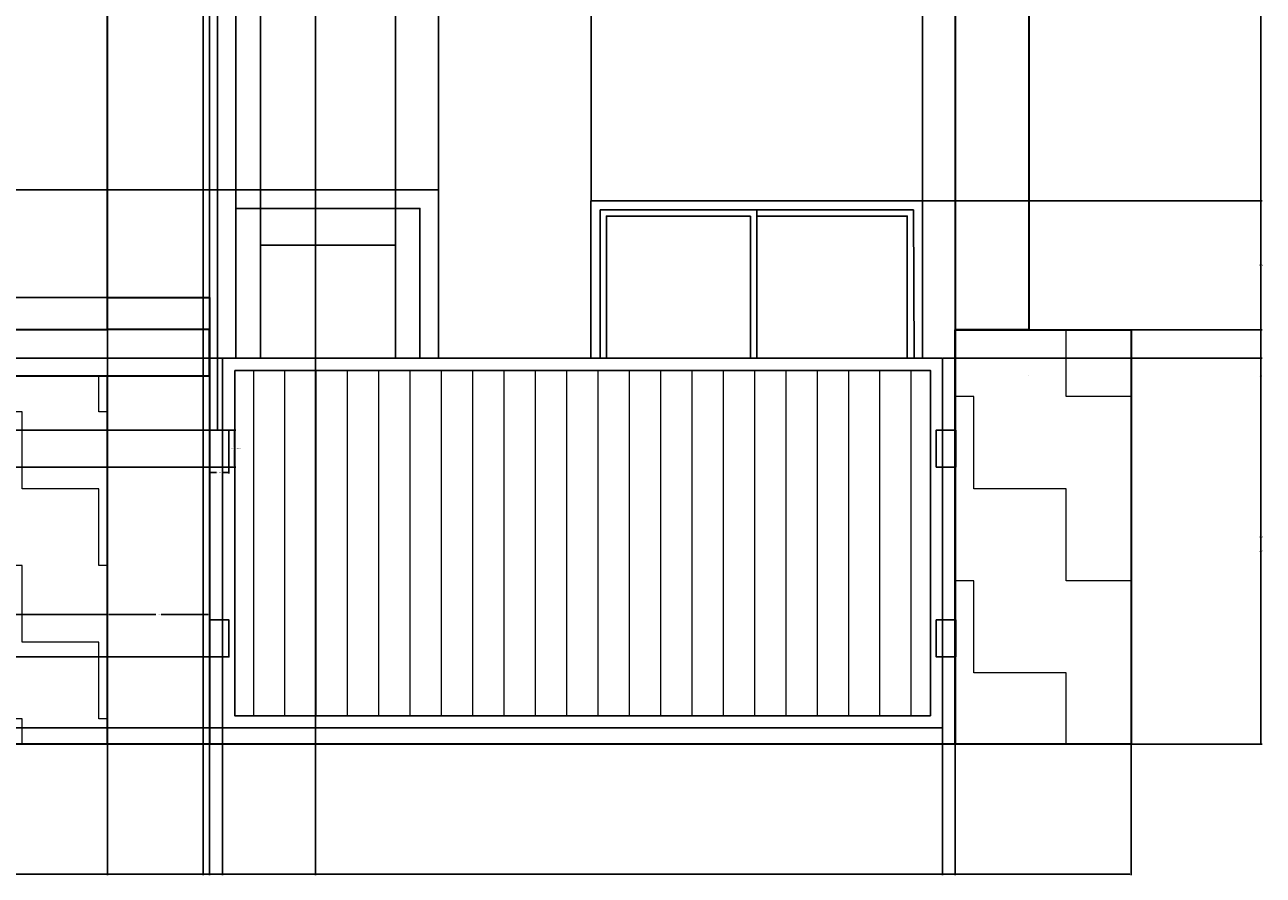
# Model space of a CAD drawing. Units: inches. Extents: x -3 to 302, y -138 to 325.
# Tile 2 of 5: x 100 to 302, y -138 to 1. Entities that reach past the tile are written whole.
import ezdxf

# ---------------------------------------------------------------- set-up
doc = ezdxf.new("R2010")
doc.units = ezdxf.units.IN
doc.header["$MEASUREMENT"] = 0
for name, color, linetype, lineweight in [('A-ANNO-DIMS', 2, 'Continuous', 18), ('A-DOOR', 4, 'Continuous', 25), ('A-ELEV', 7, 'Continuous', 35), ('A-ELEV-PATT', 8, 'Continuous', 13), ('A-GLAZ', 3, 'Continuous', 25)]:
    doc.layers.add(name, color=color, linetype=linetype, lineweight=lineweight)
doc.styles.get("Standard").update_dxf_attribs({"font": 'arial.ttf'})
doc.dimstyles.get("Standard").update_dxf_attribs({"dimtxt": 0.18, "dimasz": 0.18, "dimexe": 0.18, "dimexo": 0.0625, "dimgap": 0.09, "dimtad": 0, "dimtih": 1, "dimtoh": 1, "dimdec": 4, "dimzin": 0, "dimdsep": 46, "dimtxsty": 'Standard', "dimcen": 0.09, "dimadec": 0, "dimazin": 0, "dimtfac": 1, "dimtdec": 4, "dimtofl": 0, "dimtmove": 0, "dimatfit": 3, "dimfxl": 1, "dimtolj": 1, "dimtzin": 0, "dimarcsym": 0})

# ---------------------------------------------------------------- blocks, each defined once
blk = doc.blocks.new('GATE-HINGE')
blk.add_lwpolyline([(130.49, -65.43), (133.68, -65.43), (133.68, -71.46), (130.49, -71.46)], close=True)
blk = doc.blocks.new('*D11')
at = {"layer": 'A-ANNO-DIMS', "color": 0, "lineweight": -2, "transparency": 16777216}
for p, q in [((133.74, -65.43), (134.77, -65.43)), ((134.59, -65.61), (134.59, -68.26)), ((134.59, -71.28), (134.59, -68.62)), ((133.74, -71.46), (134.77, -71.46))]:
    blk.add_line(p, q, dxfattribs=at)
at = {"layer": 'A-ANNO-DIMS', "color": 0, "transparency": 16777216}
for points in [[(134.56, -65.61), (134.62, -65.61), (134.59, -65.43)], [(134.56, -71.28), (134.62, -71.28), (134.59, -71.46)]]:
    blk.add_solid(points, dxfattribs=at)
at = {"layer": 'Defpoints', "color": 0, "transparency": 16777216}
for p in [(133.68, -65.43), (134.59, -65.43), (133.68, -71.46)]:
    blk.add_point(p, dxfattribs=at)
at = {"layer": 'A-ANNO-DIMS', "color": 0, "transparency": 16777216, "insert": (134.59, -68.44), "char_height": 0.18, "attachment_point": 5}
blk.add_mtext('\\A1;GATE HINGE 6 TYP.', dxfattribs=at)
blk = doc.blocks.new('*D12')
at = {"layer": 'A-ANNO-DIMS', "color": 0, "lineweight": -2, "transparency": 16777216}
for p, q in [((130.49, -71.52), (130.49, -72.54)), ((130.67, -72.36), (131.63, -72.36)), ((133.5, -72.36), (132.54, -72.36)), ((133.68, -71.52), (133.68, -72.54))]:
    blk.add_line(p, q, dxfattribs=at)
at = {"layer": 'A-ANNO-DIMS', "color": 0, "transparency": 16777216}
for points in [[(130.67, -72.33), (130.67, -72.39), (130.49, -72.36)], [(133.5, -72.33), (133.5, -72.39), (133.68, -72.36)]]:
    blk.add_solid(points, dxfattribs=at)
at = {"layer": 'Defpoints', "color": 0, "transparency": 16777216}
for p in [(130.49, -71.46), (133.68, -71.46), (133.68, -72.36)]:
    blk.add_point(p, dxfattribs=at)
at = {"layer": 'A-ANNO-DIMS', "color": 0, "transparency": 16777216, "insert": (132.09, -72.36), "char_height": 0.18, "attachment_point": 5}
blk.add_mtext('\\A1;3 TYP.', dxfattribs=at)
blk = doc.blocks.new('*D17')
at = {"layer": 'A-ANNO-DIMS', "color": 0, "lineweight": -2, "transparency": 16777216}
for p, q in [((18.53, -56.69), (18.53, -137.96)), ((280.59, -116.69), (280.59, -137.96)), ((18.71, -137.78), (149.1, -137.78)), ((280.41, -137.78), (150.03, -137.78))]:
    blk.add_line(p, q, dxfattribs=at)
at = {"layer": 'A-ANNO-DIMS', "color": 0, "transparency": 16777216}
for points in [[(18.71, -137.75), (18.71, -137.81), (18.53, -137.78)], [(280.41, -137.75), (280.41, -137.81), (280.59, -137.78)]]:
    blk.add_solid(points, dxfattribs=at)
at = {"layer": 'Defpoints', "color": 0, "transparency": 16777216}
for p in [(18.53, -56.63), (280.59, -116.63), (280.59, -137.78)]:
    blk.add_point(p, dxfattribs=at)
at = {"layer": 'A-ANNO-DIMS', "color": 0, "transparency": 16777216, "insert": (149.56, -137.78), "char_height": 0.18, "attachment_point": 5}
blk.add_mtext('\\A1;262.06', dxfattribs=at)
blk = doc.blocks.new('*D19')
at = {"layer": 'A-ANNO-DIMS', "color": 0, "lineweight": -2, "transparency": 16777216}
for p, q in [((275.98, 3.37), (301.92, 3.37)), ((301.74, 3.19), (301.74, -56.44)), ((301.74, -116.45), (301.74, -56.81)), ((280.66, -116.63), (301.92, -116.63))]:
    blk.add_line(p, q, dxfattribs=at)
at = {"layer": 'A-ANNO-DIMS', "color": 0, "transparency": 16777216}
for points in [[(301.71, 3.19), (301.77, 3.19), (301.74, 3.37)], [(301.71, -116.45), (301.77, -116.45), (301.74, -116.63)]]:
    blk.add_solid(points, dxfattribs=at)
at = {"layer": 'Defpoints', "color": 0, "transparency": 16777216}
for p in [(275.92, 3.37), (301.74, 3.37), (280.59, -116.63)]:
    blk.add_point(p, dxfattribs=at)
at = {"layer": 'A-ANNO-DIMS', "color": 0, "transparency": 16777216, "insert": (301.74, -56.63), "char_height": 0.18, "attachment_point": 5}
blk.add_mtext('\\A1;120', dxfattribs=at)
blk = doc.blocks.new('*D32')
at = {"layer": 'A-ANNO-DIMS', "color": 0, "lineweight": -2, "transparency": 16777216}
for p, q in [((23.92, -116.56), (23.92, -95.3)), ((24.1, -95.48), (68.7, -95.48)), ((113.74, -95.48), (69.14, -95.48)), ((113.92, -116.56), (113.92, -95.3))]:
    blk.add_line(p, q, dxfattribs=at)
at = {"layer": 'A-ANNO-DIMS', "color": 0, "transparency": 16777216}
for points in [[(24.1, -95.45), (24.1, -95.51), (23.92, -95.48)], [(113.74, -95.45), (113.74, -95.51), (113.92, -95.48)]]:
    blk.add_solid(points, dxfattribs=at)
at = {"layer": 'Defpoints', "color": 0, "transparency": 16777216}
for p in [(113.92, -95.48), (23.92, -116.63), (113.92, -116.63)]:
    blk.add_point(p, dxfattribs=at)
at = {"layer": 'A-ANNO-DIMS', "color": 0, "transparency": 16777216, "insert": (68.92, -95.48), "char_height": 0.18, "attachment_point": 5}
blk.add_mtext('\\A1;90', dxfattribs=at)
blk = doc.blocks.new('*D33')
at = {"layer": 'A-ANNO-DIMS', "color": 0, "lineweight": -2, "transparency": 16777216}
for p, q in [((113.92, -116.56), (113.92, -95.3)), ((114.1, -95.48), (121.75, -95.48)), ((130.31, -95.48), (122.66, -95.48)), ((130.49, -116.56), (130.49, -95.3))]:
    blk.add_line(p, q, dxfattribs=at)
at = {"layer": 'A-ANNO-DIMS', "color": 0, "transparency": 16777216}
for points in [[(114.1, -95.45), (114.1, -95.51), (113.92, -95.48)], [(130.31, -95.45), (130.31, -95.51), (130.49, -95.48)]]:
    blk.add_solid(points, dxfattribs=at)
at = {"layer": 'Defpoints', "color": 0, "transparency": 16777216}
for p in [(130.49, -95.48), (113.92, -116.63), (130.49, -116.63)]:
    blk.add_point(p, dxfattribs=at)
at = {"layer": 'A-ANNO-DIMS', "color": 0, "transparency": 16777216, "insert": (122.21, -95.48), "char_height": 0.18, "attachment_point": 5}
blk.add_mtext('\\A1;16.567', dxfattribs=at)
blk = doc.blocks.new('*D66')
at = {"layer": 'A-ANNO-DIMS', "color": 0, "lineweight": -2, "transparency": 16777216}
for p, q in [((113.92, 141.31), (113.92, -137.96)), ((129.47, 141.31), (129.47, -137.96)), ((114.1, -137.78), (121.24, -137.78)), ((129.29, -137.78), (122.15, -137.78))]:
    blk.add_line(p, q, dxfattribs=at)
at = {"layer": 'A-ANNO-DIMS', "color": 0, "transparency": 16777216}
for points in [[(114.1, -137.75), (114.1, -137.81), (113.92, -137.78)], [(129.29, -137.75), (129.29, -137.81), (129.47, -137.78)]]:
    blk.add_solid(points, dxfattribs=at)
at = {"layer": 'Defpoints', "color": 0, "transparency": 16777216}
for p in [(113.92, 141.37), (129.47, 141.37), (129.47, -137.78)]:
    blk.add_point(p, dxfattribs=at)
at = {"layer": 'A-ANNO-DIMS', "color": 0, "transparency": 16777216, "insert": (121.7, -137.78), "char_height": 0.18, "attachment_point": 5}
blk.add_mtext('\\A1;15.553', dxfattribs=at)
blk = doc.blocks.new('*D67')
at = {"layer": 'A-ANNO-DIMS', "color": 0, "lineweight": -2, "transparency": 16777216}
for p, q in [((129.47, 141.31), (129.47, -137.96)), ((147.75, 141.31), (147.75, -137.96)), ((129.65, -137.78), (138.16, -137.78)), ((147.57, -137.78), (139.07, -137.78))]:
    blk.add_line(p, q, dxfattribs=at)
at = {"layer": 'A-ANNO-DIMS', "color": 0, "transparency": 16777216}
for points in [[(129.65, -137.75), (129.65, -137.81), (129.47, -137.78)], [(147.57, -137.75), (147.57, -137.81), (147.75, -137.78)]]:
    blk.add_solid(points, dxfattribs=at)
at = {"layer": 'Defpoints', "color": 0, "transparency": 16777216}
for p in [(129.47, 141.37), (147.75, 141.37), (147.75, -137.78)]:
    blk.add_point(p, dxfattribs=at)
at = {"layer": 'A-ANNO-DIMS', "color": 0, "transparency": 16777216, "insert": (138.61, -137.78), "char_height": 0.18, "attachment_point": 5}
blk.add_mtext('\\A1;18.274', dxfattribs=at)
blk = doc.blocks.new('*D68')
at = {"layer": 'A-ANNO-DIMS', "color": 0, "lineweight": -2, "transparency": 16777216}
for p, q in [((130.489456, -43.793388), (130.489456, 324.704711)), ((130.669456, 324.524711), (130.823276, 324.524711)), ((131.607096, 324.524711), (131.453276, 324.524711)), ((131.787096, -26.240874), (131.787096, 324.704711))]:
    blk.add_line(p, q, dxfattribs=at)
at = {"layer": 'A-ANNO-DIMS', "color": 0, "transparency": 16777216}
for points in [[(130.669456, 324.554711), (130.669456, 324.494711), (130.489456, 324.524711)], [(131.607096, 324.554711), (131.607096, 324.494711), (131.787096, 324.524711)]]:
    blk.add_solid(points, dxfattribs=at)
at = {"layer": 'Defpoints', "color": 0, "transparency": 16777216}
for p in [(131.787096, 324.524711), (131.787096, -26.303374), (130.489456, -43.855888)]:
    blk.add_point(p, dxfattribs=at)
at = {"layer": 'A-ANNO-DIMS', "color": 0, "transparency": 16777216, "insert": (131.138276, 324.524711), "char_height": 0.18, "attachment_point": 5}
blk.add_mtext('\\A1;1.30', dxfattribs=at)
blk = doc.blocks.new('*D69')
at = {"layer": 'A-ANNO-DIMS', "color": 0, "lineweight": -2, "transparency": 16777216}
for p, q in [((131.79, -26.24), (131.79, 324.7)), ((131.97, 324.52), (149.57, 324.52)), ((167.61, 324.52), (150.01, 324.52)), ((167.79, -26.24), (167.79, 324.7))]:
    blk.add_line(p, q, dxfattribs=at)
at = {"layer": 'A-ANNO-DIMS', "color": 0, "transparency": 16777216}
for points in [[(131.97, 324.55), (131.97, 324.49), (131.79, 324.52)], [(167.61, 324.55), (167.61, 324.49), (167.79, 324.52)]]:
    blk.add_solid(points, dxfattribs=at)
at = {"layer": 'Defpoints', "color": 0, "transparency": 16777216}
for p in [(167.79, 324.52), (131.79, -26.3), (167.79, -26.3)]:
    blk.add_point(p, dxfattribs=at)
at = {"layer": 'A-ANNO-DIMS', "color": 0, "transparency": 16777216, "insert": (149.79, 324.52), "char_height": 0.18, "attachment_point": 5}
blk.add_mtext('\\A1;36', dxfattribs=at)
blk = doc.blocks.new('*D70')
at = {"layer": 'A-ANNO-DIMS', "color": 0, "lineweight": -2, "transparency": 16777216}
for p, q in [((167.79, -26.24), (167.79, 324.7)), ((167.97, 324.52), (179.82, 324.52)), ((192.46, 324.52), (180.61, 324.52)), ((192.64, -28.02), (192.64, 324.7))]:
    blk.add_line(p, q, dxfattribs=at)
at = {"layer": 'A-ANNO-DIMS', "color": 0, "transparency": 16777216}
for points in [[(167.97, 324.55), (167.97, 324.49), (167.79, 324.52)], [(192.46, 324.55), (192.46, 324.49), (192.64, 324.52)]]:
    blk.add_solid(points, dxfattribs=at)
at = {"layer": 'Defpoints', "color": 0, "transparency": 16777216}
for p in [(192.64, 324.52), (167.79, -26.3), (192.64, -28.09)]:
    blk.add_point(p, dxfattribs=at)
at = {"layer": 'A-ANNO-DIMS', "color": 0, "transparency": 16777216, "insert": (180.21, 324.52), "char_height": 0.18, "attachment_point": 5}
blk.add_mtext('\\A1;24.85', dxfattribs=at)
blk = doc.blocks.new('*D71')
at = {"layer": 'A-ANNO-DIMS', "color": 0, "lineweight": -2, "transparency": 16777216}
for p, q in [((192.64, -28.02), (192.64, 324.7)), ((192.82, 324.52), (219.42, 324.52)), ((246.46, 324.52), (219.86, 324.52)), ((246.64, -28.02), (246.64, 324.7))]:
    blk.add_line(p, q, dxfattribs=at)
at = {"layer": 'A-ANNO-DIMS', "color": 0, "transparency": 16777216}
for points in [[(192.82, 324.55), (192.82, 324.49), (192.64, 324.52)], [(246.46, 324.55), (246.46, 324.49), (246.64, 324.52)]]:
    blk.add_solid(points, dxfattribs=at)
at = {"layer": 'Defpoints', "color": 0, "transparency": 16777216}
for p in [(246.64, 324.52), (192.64, -28.09), (246.64, -28.09)]:
    blk.add_point(p, dxfattribs=at)
at = {"layer": 'A-ANNO-DIMS', "color": 0, "transparency": 16777216, "insert": (219.64, 324.52), "char_height": 0.18, "attachment_point": 5}
blk.add_mtext('\\A1;54', dxfattribs=at)
blk = doc.blocks.new('*D72')
at = {"layer": 'A-ANNO-DIMS', "color": 0, "lineweight": -2, "transparency": 16777216}
for p, q in [((246.64, -28.02), (246.64, 324.7)), ((246.82, 324.52), (248.89, 324.52)), ((251.74, 324.52), (249.67, 324.52)), ((251.92, -49.03), (251.92, 324.7))]:
    blk.add_line(p, q, dxfattribs=at)
at = {"layer": 'A-ANNO-DIMS', "color": 0, "transparency": 16777216}
for points in [[(246.82, 324.55), (246.82, 324.49), (246.64, 324.52)], [(251.74, 324.55), (251.74, 324.49), (251.92, 324.52)]]:
    blk.add_solid(points, dxfattribs=at)
at = {"layer": 'Defpoints', "color": 0, "transparency": 16777216}
for p in [(251.92, 324.52), (246.64, -28.09), (251.92, -49.09)]:
    blk.add_point(p, dxfattribs=at)
at = {"layer": 'A-ANNO-DIMS', "color": 0, "transparency": 16777216, "insert": (249.28, 324.52), "char_height": 0.18, "attachment_point": 5}
blk.add_mtext('\\A1;5.285', dxfattribs=at)
blk = doc.blocks.new('*D73')
at = {"layer": 'A-ANNO-DIMS', "color": 0, "lineweight": -2, "transparency": 16777216}
for p, q in [((131.79, -26.24), (131.79, 324.7)), ((131.97, 324.52), (133.14, 324.52)), ((134.61, 324.52), (133.44, 324.52)), ((134.79, -29.26), (134.79, 324.7))]:
    blk.add_line(p, q, dxfattribs=at)
at = {"layer": 'A-ANNO-DIMS', "color": 0, "transparency": 16777216}
for points in [[(131.97, 324.55), (131.97, 324.49), (131.79, 324.52)], [(134.61, 324.55), (134.61, 324.49), (134.79, 324.52)]]:
    blk.add_solid(points, dxfattribs=at)
at = {"layer": 'Defpoints', "color": 0, "transparency": 16777216}
for p in [(134.79, 324.52), (131.79, -26.3), (134.79, -29.33)]:
    blk.add_point(p, dxfattribs=at)
at = {"layer": 'A-ANNO-DIMS', "color": 0, "transparency": 16777216, "insert": (133.29, 324.52), "char_height": 0.18, "attachment_point": 5}
blk.add_mtext('\\A1;3', dxfattribs=at)
blk = doc.blocks.new('*D74')
at = {"layer": 'A-ANNO-DIMS', "color": 0, "lineweight": -2, "transparency": 16777216}
for p, q in [((134.79, -29.26), (134.79, 324.7)), ((134.97, 324.52), (136.63, 324.52)), ((138.61, 324.52), (136.94, 324.52)), ((138.79, -35.26), (138.79, 324.7))]:
    blk.add_line(p, q, dxfattribs=at)
at = {"layer": 'A-ANNO-DIMS', "color": 0, "transparency": 16777216}
for points in [[(134.97, 324.55), (134.97, 324.49), (134.79, 324.52)], [(138.61, 324.55), (138.61, 324.49), (138.79, 324.52)]]:
    blk.add_solid(points, dxfattribs=at)
at = {"layer": 'Defpoints', "color": 0, "transparency": 16777216}
for p in [(138.79, 324.52), (134.79, -29.33), (138.79, -35.33)]:
    blk.add_point(p, dxfattribs=at)
at = {"layer": 'A-ANNO-DIMS', "color": 0, "transparency": 16777216, "insert": (136.79, 324.52), "char_height": 0.18, "attachment_point": 5}
blk.add_mtext('\\A1;4', dxfattribs=at)
blk = doc.blocks.new('*D75')
at = {"layer": 'A-ANNO-DIMS', "color": 0, "lineweight": -2, "transparency": 16777216}
for p, q in [((138.79, -35.26), (138.79, 324.7)), ((138.97, 324.52), (149.57, 324.52)), ((160.61, 324.52), (150.01, 324.52)), ((160.79, -35.26), (160.79, 324.7))]:
    blk.add_line(p, q, dxfattribs=at)
at = {"layer": 'A-ANNO-DIMS', "color": 0, "transparency": 16777216}
for points in [[(138.97, 324.55), (138.97, 324.49), (138.79, 324.52)], [(160.61, 324.55), (160.61, 324.49), (160.79, 324.52)]]:
    blk.add_solid(points, dxfattribs=at)
at = {"layer": 'Defpoints', "color": 0, "transparency": 16777216}
for p in [(160.79, 324.52), (138.79, -35.33), (160.79, -35.33)]:
    blk.add_point(p, dxfattribs=at)
at = {"layer": 'A-ANNO-DIMS', "color": 0, "transparency": 16777216, "insert": (149.79, 324.52), "char_height": 0.18, "attachment_point": 5}
blk.add_mtext('\\A1;22', dxfattribs=at)
blk = doc.blocks.new('*D76')
at = {"layer": 'A-ANNO-DIMS', "color": 0, "lineweight": -2, "transparency": 16777216}
for p, q in [((132.57, -113.96), (-2.8, -113.96)), ((-2.62, -114.14), (-2.62, -115.11)), ((130.43, -116.63), (-2.8, -116.63)), ((-2.62, -116.45), (-2.62, -115.48))]:
    blk.add_line(p, q, dxfattribs=at)
at = {"layer": 'A-ANNO-DIMS', "color": 0, "transparency": 16777216}
for points in [[(-2.65, -114.14), (-2.59, -114.14), (-2.62, -113.96)], [(-2.65, -116.45), (-2.59, -116.45), (-2.62, -116.63)]]:
    blk.add_solid(points, dxfattribs=at)
at = {"layer": 'Defpoints', "color": 0, "transparency": 16777216}
for p in [(-2.62, -113.96), (132.63, -113.96), (130.49, -116.63)]:
    blk.add_point(p, dxfattribs=at)
at = {"layer": 'A-ANNO-DIMS', "color": 0, "transparency": 16777216, "insert": (-2.62, -115.29), "char_height": 0.18, "attachment_point": 5}
blk.add_mtext('\\A1;2.661', dxfattribs=at)
blk = doc.blocks.new('*D77')
at = {"layer": 'A-ANNO-DIMS', "color": 0, "lineweight": -2, "transparency": 16777216}
for p, q in [((130.43, -102.38), (-2.8, -102.38)), ((-2.62, -102.56), (-2.62, -107.99)), ((-2.62, -113.78), (-2.62, -108.36)), ((132.57, -113.96), (-2.8, -113.96))]:
    blk.add_line(p, q, dxfattribs=at)
at = {"layer": 'A-ANNO-DIMS', "color": 0, "transparency": 16777216}
for points in [[(-2.65, -102.56), (-2.59, -102.56), (-2.62, -102.38)], [(-2.65, -113.78), (-2.59, -113.78), (-2.62, -113.96)]]:
    blk.add_solid(points, dxfattribs=at)
at = {"layer": 'Defpoints', "color": 0, "transparency": 16777216}
for p in [(-2.62, -102.38), (130.49, -102.38), (132.63, -113.96)]:
    blk.add_point(p, dxfattribs=at)
at = {"layer": 'A-ANNO-DIMS', "color": 0, "transparency": 16777216, "insert": (-2.62, -108.17), "char_height": 0.18, "attachment_point": 5}
blk.add_mtext('\\A1;11.582', dxfattribs=at)
blk = doc.blocks.new('*D78')
at = {"layer": 'A-ANNO-DIMS', "color": 0, "lineweight": -2, "transparency": 16777216}
for p, q in [((130.43, -71.46), (-2.8, -71.46)), ((-2.62, -71.64), (-2.62, -86.74)), ((-2.62, -102.2), (-2.62, -87.1)), ((130.43, -102.38), (-2.8, -102.38))]:
    blk.add_line(p, q, dxfattribs=at)
at = {"layer": 'A-ANNO-DIMS', "color": 0, "transparency": 16777216}
for points in [[(-2.65, -71.64), (-2.59, -71.64), (-2.62, -71.46)], [(-2.65, -102.2), (-2.59, -102.2), (-2.62, -102.38)]]:
    blk.add_solid(points, dxfattribs=at)
at = {"layer": 'Defpoints', "color": 0, "transparency": 16777216}
for p in [(-2.62, -71.46), (130.49, -71.46), (130.49, -102.38)]:
    blk.add_point(p, dxfattribs=at)
at = {"layer": 'A-ANNO-DIMS', "color": 0, "transparency": 16777216, "insert": (-2.62, -86.92), "char_height": 0.18, "attachment_point": 5}
blk.add_mtext('\\A1;30.926', dxfattribs=at)
blk = doc.blocks.new('*D79')
at = {"layer": 'A-ANNO-DIMS', "color": 0, "lineweight": -2, "transparency": 16777216}
for p, q in [((132.57, -53.73), (-2.8, -53.73)), ((-2.62, -53.91), (-2.62, -59.4)), ((-2.62, -65.25), (-2.62, -59.76)), ((130.43, -65.43), (-2.8, -65.43))]:
    blk.add_line(p, q, dxfattribs=at)
at = {"layer": 'A-ANNO-DIMS', "color": 0, "transparency": 16777216}
for points in [[(-2.65, -53.91), (-2.59, -53.91), (-2.62, -53.73)], [(-2.65, -65.25), (-2.59, -65.25), (-2.62, -65.43)]]:
    blk.add_solid(points, dxfattribs=at)
at = {"layer": 'Defpoints', "color": 0, "transparency": 16777216}
for p in [(-2.62, -53.73), (132.63, -53.73), (130.49, -65.43)]:
    blk.add_point(p, dxfattribs=at)
at = {"layer": 'A-ANNO-DIMS', "color": 0, "transparency": 16777216, "insert": (-2.62, -59.58), "char_height": 0.18, "attachment_point": 5}
blk.add_mtext('\\A1;11.695', dxfattribs=at)
blk = doc.blocks.new('*D80')
at = {"layer": 'A-ANNO-DIMS', "color": 0, "lineweight": -2, "transparency": 16777216}
for p, q in [((130.43, -43.86), (-2.8, -43.86)), ((-2.62, -44.04), (-2.62, -48.61)), ((-2.62, -53.55), (-2.62, -48.98)), ((132.57, -53.73), (-2.8, -53.73))]:
    blk.add_line(p, q, dxfattribs=at)
at = {"layer": 'A-ANNO-DIMS', "color": 0, "transparency": 16777216}
for points in [[(-2.65, -44.04), (-2.59, -44.04), (-2.62, -43.86)], [(-2.65, -53.55), (-2.59, -53.55), (-2.62, -53.73)]]:
    blk.add_solid(points, dxfattribs=at)
at = {"layer": 'Defpoints', "color": 0, "transparency": 16777216}
for p in [(-2.62, -43.86), (130.49, -43.86), (132.63, -53.73)]:
    blk.add_point(p, dxfattribs=at)
at = {"layer": 'A-ANNO-DIMS', "color": 0, "transparency": 16777216, "insert": (-2.62, -48.79), "char_height": 0.18, "attachment_point": 5}
blk.add_mtext('\\A1;9.876', dxfattribs=at)
blk = doc.blocks.new('*D81')
at = {"layer": 'A-ANNO-DIMS', "color": 0, "lineweight": -2, "transparency": 16777216}
for p, q in [((131.72, -26.3), (-2.8, -26.3)), ((-2.62, -26.48), (-2.62, -34.9)), ((-2.62, -43.68), (-2.62, -35.26)), ((130.43, -43.86), (-2.8, -43.86))]:
    blk.add_line(p, q, dxfattribs=at)
at = {"layer": 'A-ANNO-DIMS', "color": 0, "transparency": 16777216}
for points in [[(-2.65, -26.48), (-2.59, -26.48), (-2.62, -26.3)], [(-2.65, -43.68), (-2.59, -43.68), (-2.62, -43.86)]]:
    blk.add_solid(points, dxfattribs=at)
at = {"layer": 'Defpoints', "color": 0, "transparency": 16777216}
for p in [(-2.62, -26.3), (131.79, -26.3), (130.49, -43.86)]:
    blk.add_point(p, dxfattribs=at)
at = {"layer": 'A-ANNO-DIMS', "color": 0, "transparency": 16777216, "insert": (-2.62, -35.08), "char_height": 0.18, "attachment_point": 5}
blk.add_mtext('\\A1;17.553', dxfattribs=at)
blk = doc.blocks.new('*D82')
at = {"layer": 'A-ANNO-DIMS', "color": 0, "lineweight": -2, "transparency": 16777216}
for p, q in [((132.63, -114.03), (132.63, -137.96)), ((130.49, -116.69), (130.49, -137.96)), ((130.67, -137.78), (131.24, -137.78)), ((132.45, -137.78), (131.89, -137.78))]:
    blk.add_line(p, q, dxfattribs=at)
at = {"layer": 'A-ANNO-DIMS', "color": 0, "transparency": 16777216}
for points in [[(130.67, -137.75), (130.67, -137.81), (130.49, -137.78)], [(132.45, -137.75), (132.45, -137.81), (132.63, -137.78)]]:
    blk.add_solid(points, dxfattribs=at)
at = {"layer": 'Defpoints', "color": 0, "transparency": 16777216}
for p in [(132.63, -113.96), (130.49, -116.63), (132.63, -137.78)]:
    blk.add_point(p, dxfattribs=at)
at = {"layer": 'A-ANNO-DIMS', "color": 0, "transparency": 16777216, "insert": (131.56, -137.78), "char_height": 0.18, "attachment_point": 5}
blk.add_mtext('\\A1;2.14', dxfattribs=at)
blk = doc.blocks.new('*D83')
at = {"layer": 'A-ANNO-DIMS', "color": 0, "lineweight": -2, "transparency": 16777216}
for p, q in [((132.63, -114.03), (132.63, -137.96)), ((249.91, -114.03), (249.91, -137.96)), ((132.81, -137.78), (190.82, -137.78)), ((249.73, -137.78), (191.73, -137.78))]:
    blk.add_line(p, q, dxfattribs=at)
at = {"layer": 'A-ANNO-DIMS', "color": 0, "transparency": 16777216}
for points in [[(132.81, -137.75), (132.81, -137.81), (132.63, -137.78)], [(249.73, -137.75), (249.73, -137.81), (249.91, -137.78)]]:
    blk.add_solid(points, dxfattribs=at)
at = {"layer": 'Defpoints', "color": 0, "transparency": 16777216}
for p in [(132.63, -113.96), (249.91, -113.96), (249.91, -137.78)]:
    blk.add_point(p, dxfattribs=at)
at = {"layer": 'A-ANNO-DIMS', "color": 0, "transparency": 16777216, "insert": (191.27, -137.78), "char_height": 0.18, "attachment_point": 5}
blk.add_mtext('\\A1;117.28', dxfattribs=at)
blk = doc.blocks.new('*D84')
at = {"layer": 'A-ANNO-DIMS', "color": 0, "lineweight": -2, "transparency": 16777216}
for p, q in [((249.91, -114.03), (249.91, -137.96)), ((251.92, -116.69), (251.92, -137.96)), ((250.09, -137.78), (250.61, -137.78)), ((251.74, -137.78), (251.22, -137.78))]:
    blk.add_line(p, q, dxfattribs=at)
at = {"layer": 'A-ANNO-DIMS', "color": 0, "transparency": 16777216}
for points in [[(250.09, -137.75), (250.09, -137.81), (249.91, -137.78)], [(251.74, -137.75), (251.74, -137.81), (251.92, -137.78)]]:
    blk.add_solid(points, dxfattribs=at)
at = {"layer": 'Defpoints', "color": 0, "transparency": 16777216}
for p in [(249.91, -113.96), (251.92, -116.63), (251.92, -137.78)]:
    blk.add_point(p, dxfattribs=at)
at = {"layer": 'A-ANNO-DIMS', "color": 0, "transparency": 16777216, "insert": (250.92, -137.78), "char_height": 0.18, "attachment_point": 5}
blk.add_mtext('\\A1;2.01', dxfattribs=at)
blk = doc.blocks.new('*D85')
at = {"layer": 'A-ANNO-DIMS', "color": 0, "lineweight": -2, "transparency": 16777216}
for p, q in [((251.92, -116.69), (251.92, -137.96)), ((280.59, -116.69), (280.59, -137.96)), ((252.1, -137.78), (265.86, -137.78)), ((280.41, -137.78), (266.65, -137.78))]:
    blk.add_line(p, q, dxfattribs=at)
at = {"layer": 'A-ANNO-DIMS', "color": 0, "transparency": 16777216}
for points in [[(252.1, -137.75), (252.1, -137.81), (251.92, -137.78)], [(280.41, -137.75), (280.41, -137.81), (280.59, -137.78)]]:
    blk.add_solid(points, dxfattribs=at)
at = {"layer": 'Defpoints', "color": 0, "transparency": 16777216}
for p in [(251.92, -116.63), (280.59, -116.63), (280.59, -137.78)]:
    blk.add_point(p, dxfattribs=at)
at = {"layer": 'A-ANNO-DIMS', "color": 0, "transparency": 16777216, "insert": (266.26, -137.78), "char_height": 0.18, "attachment_point": 5}
blk.add_mtext('\\A1;28.67', dxfattribs=at)
blk = doc.blocks.new('*D86')
at = {"layer": 'A-ANNO-DIMS', "color": 0, "lineweight": -2, "transparency": 16777216}
for p, q in [((249.97, -53.73), (301.92, -53.73)), ((301.74, -53.91), (301.74, -85)), ((301.74, -116.45), (301.74, -85.36)), ((251.98, -116.63), (301.92, -116.63))]:
    blk.add_line(p, q, dxfattribs=at)
at = {"layer": 'A-ANNO-DIMS', "color": 0, "transparency": 16777216}
for points in [[(301.71, -53.91), (301.77, -53.91), (301.74, -53.73)], [(301.71, -116.45), (301.77, -116.45), (301.74, -116.63)]]:
    blk.add_solid(points, dxfattribs=at)
at = {"layer": 'Defpoints', "color": 0, "transparency": 16777216}
for p in [(249.91, -53.73), (301.74, -53.73), (251.92, -116.63)]:
    blk.add_point(p, dxfattribs=at)
at = {"layer": 'A-ANNO-DIMS', "color": 0, "transparency": 16777216, "insert": (301.74, -85.18), "char_height": 0.18, "attachment_point": 5}
blk.add_mtext('\\A1;62.89', dxfattribs=at)
blk = doc.blocks.new('*D87')
at = {"layer": 'A-ANNO-DIMS', "color": 0, "lineweight": -2, "transparency": 16777216}
for p, q in [((280.66, -49.09), (301.92, -49.09)), ((301.74, -49.27), (301.74, -82.68)), ((301.74, -116.45), (301.74, -83.04)), ((280.66, -116.63), (301.92, -116.63))]:
    blk.add_line(p, q, dxfattribs=at)
at = {"layer": 'A-ANNO-DIMS', "color": 0, "transparency": 16777216}
for points in [[(301.71, -49.27), (301.77, -49.27), (301.74, -49.09)], [(301.71, -116.45), (301.77, -116.45), (301.74, -116.63)]]:
    blk.add_solid(points, dxfattribs=at)
at = {"layer": 'Defpoints', "color": 0, "transparency": 16777216}
for p in [(280.59, -49.09), (301.74, -49.09), (280.59, -116.63)]:
    blk.add_point(p, dxfattribs=at)
at = {"layer": 'A-ANNO-DIMS', "color": 0, "transparency": 16777216, "insert": (301.74, -82.86), "char_height": 0.18, "attachment_point": 5}
blk.add_mtext('\\A1;67.53', dxfattribs=at)
blk = doc.blocks.new('*D88')
at = {"layer": 'A-ANNO-DIMS', "color": 0, "lineweight": -2, "transparency": 16777216}
for p, q in [((246.7, -28.09), (301.92, -28.09)), ((301.74, -28.27), (301.74, -38.41)), ((301.74, -48.91), (301.74, -38.77)), ((263.98, -49.09), (301.92, -49.09))]:
    blk.add_line(p, q, dxfattribs=at)
at = {"layer": 'A-ANNO-DIMS', "color": 0, "transparency": 16777216}
for points in [[(301.71, -28.27), (301.77, -28.27), (301.74, -28.09)], [(301.71, -48.91), (301.77, -48.91), (301.74, -49.09)]]:
    blk.add_solid(points, dxfattribs=at)
at = {"layer": 'Defpoints', "color": 0, "transparency": 16777216}
for p in [(246.64, -28.09), (301.74, -28.09), (263.92, -49.09)]:
    blk.add_point(p, dxfattribs=at)
at = {"layer": 'A-ANNO-DIMS', "color": 0, "transparency": 16777216, "insert": (301.74, -38.59), "char_height": 0.18, "attachment_point": 5}
blk.add_mtext('\\A1;21.006', dxfattribs=at)

msp = doc.modelspace()

# ---------------------------------------------------------------- hatches: boundary and pattern name
at = {"layer": 'A-ELEV-PATT'}
h = msp.add_hatch(dxfattribs=at)
h.set_pattern_fill('ZIGZAG', color=256, scale=120, angle=90)
h.set_pattern_definition([(90, (0, 0), (-15, 15), [15, -15]), (180, (9e-16, 15), (-15, -15), [15, -15])])
h.paths.add_polyline_path([(280.5936, -49.0923), (251.922, -49.0923), (251.922, -65.4264), (252.0519, -65.4264), (252.0519, -71.4563), (251.9803, -96.3528), (252.0519, -96.3528), (252.0519, -102.3827), (251.922, -116.6253), (280.5936, -116.6253)])
h = msp.add_hatch(dxfattribs=at)
h.set_pattern_fill('_USER', color=256, scale=5.1, angle=90, pattern_type=0)
h.set_pattern_definition([(90, (0, 0), (-5.1, 3e-16), [])])
h.paths.add_polyline_path([(247.9086, -55.7317), (134.6328, -55.7317), (134.6328, -111.9645), (247.9086, -111.9645)])
h = msp.add_hatch(dxfattribs=at)
h.set_pattern_fill('ZIGZAG', color=256, scale=100, angle=90)
h.set_pattern_definition([(90, (0, 0), (-12.5, 12.5), [12.5, -12.5]), (180, (8e-16, 12.5), (-12.5, -12.5), [12.5, -12.5])])
h.paths.add_polyline_path([(113.922, -56.6253), (23.922, -56.6253), (23.922, -116.6253), (113.922, -116.6253)])

# ---------------------------------------------------------------- linework, layer by layer
at = {"layer": 'A-DOOR'}
for points in [[(131.7871, -65.4264), (131.7871, -26.3034), (167.7871, -26.3034), (167.7871, -53.7317)], [(134.7871, -53.7317), (134.7871, -29.3264), (164.7871, -29.3264), (164.7871, -53.7317)], [(160.7871, -53.7317), (160.7871, -35.3264), (138.7871, -35.3264), (138.7871, -53.7317)]]:
    msp.add_lwpolyline(points, dxfattribs=at)
for points in [[(132.6328, -53.7317), (249.9086, -53.7317), (249.9086, -113.9645), (132.6328, -113.9645)], [(134.6328, -55.7317), (247.9086, -55.7317), (247.9086, -111.9645), (134.6328, -111.9645)]]:
    msp.add_lwpolyline(points, close=True, dxfattribs=at)
at = {"layer": 'A-ELEV'}
for p, q in [((113.922, -49.0923), (113.922, 3.3747)), ((251.922, 3.3747), (251.922, -116.6253)), ((263.922, 3.3747), (263.922, -49.0923)), ((23.922, -56.6253), (113.922, -56.6253)), ((113.922, -116.6253), (113.922, -56.6253)), ((263.922, -116.6253), (23.922, -116.6253))]:
    msp.add_line(p, q, dxfattribs=at)
for points in [[(113.922, -49.0923), (113.922, -43.8559), (130.4895, -43.8559), (130.4895, -116.6253), (113.922, -116.6253), (113.922, -56.6253)], [(113.922, -49.0923), (18.5303, -49.0923), (18.5303, -56.6253), (113.922, -56.6253)], [(113.922, -56.6253), (130.4895, -56.6253), (130.4895, -49.0797), (113.922, -49.0797), (113.922, -49.0923)], [(263.922, -49.0923), (251.922, -49.0923)]]:
    msp.add_lwpolyline(points, dxfattribs=at)
for points in [[(251.922, -49.0923), (280.5936, -49.0923), (280.5936, -116.6253), (251.922, -116.6253)], [(263.922, -56.6253), (263.922, -56.6253)]]:
    msp.add_lwpolyline(points, close=True, dxfattribs=at)
at = {"layer": 'A-GLAZ'}
for p, q in [((194.1368, -29.5862), (219.6368, -29.5862)), ((194.1368, -53.7317), (194.1368, -29.5862)), ((219.6368, -29.5862), (245.1368, -29.5862)), ((219.6368, -53.7317), (219.6368, -29.5862)), ((245.1368, -29.5862), (245.2586, -53.7317))]:
    msp.add_line(p, q, dxfattribs=at)
for points in [[(192.6368, -53.7317), (192.6368, -28.0862), (246.6368, -28.0862), (246.6368, -53.7317)], [(195.1368, -53.7317), (195.1368, -30.5862), (218.6368, -30.5862)], [(218.6368, -30.5861), (218.6368, -53.7317)], [(219.6368, -30.5862), (244.1368, -30.5862), (244.1368, -53.7317)]]:
    msp.add_lwpolyline(points, dxfattribs=at)

# ---------------------------------------------------------------- block references
at = {"layer": 'A-DOOR'}
for p in [(0, 0), (0, -30.9264)]:
    msp.add_blockref('GATE-HINGE', p, dxfattribs=at)
at = {"layer": 'A-DOOR', "extrusion": (0, 0, -1), "zscale": -1}
for p in [(-382.5413, 0), (-382.5413, -30.9264)]:
    msp.add_blockref('GATE-HINGE', p, dxfattribs=at)

# ---------------------------------------------------------------- dimensions: what is measured, and where the dimension line sits
at = {"layer": 'A-ANNO-DIMS'}
for base, p1, p2, override, picture, middle in [((131.7871, 324.5247), (130.4895, -43.8559), (131.7871, -26.3034), {"dimdec": 2, "dimlfac": 1, "dimrnd": 0, "dimzin": 0, "dimdsep": 46, "dimlunit": 2}, '*D68', (131.1383, 324.5247)), ((167.7871, 324.5247), (131.7871, -26.3034), (167.7871, -26.3034), {"dimdec": 0, "dimlfac": 1, "dimrnd": 0, "dimzin": 0, "dimdsep": 46, "dimlunit": 2}, '*D69', (149.7871, 324.5247)), ((134.7871, 324.5247), (131.7871, -26.3034), (134.7871, -29.3264), {"dimdec": 0, "dimlfac": 1, "dimrnd": 0, "dimzin": 0, "dimdsep": 46, "dimlunit": 2}, '*D73', (133.2871, 324.5247)), ((138.7871, 324.5247), (134.7871, -29.3264), (138.7871, -35.3264), {"dimdec": 0, "dimlfac": 1, "dimrnd": 0, "dimzin": 0, "dimdsep": 46, "dimlunit": 2}, '*D74', (136.7871, 324.5247)), ((160.7871, 324.5247), (138.7871, -35.3264), (160.7871, -35.3264), {"dimdec": 0, "dimlfac": 1, "dimrnd": 0, "dimzin": 0, "dimdsep": 46, "dimlunit": 2}, '*D75', (149.7871, 324.5247)), ((192.6368, 324.5247), (167.7871, -26.3034), (192.6368, -28.0862), {"dimdec": 2, "dimlfac": 1, "dimrnd": 0, "dimzin": 0, "dimdsep": 46, "dimlunit": 2}, '*D70', (180.2119, 324.5247)), ((246.6368, 324.5247), (192.6368, -28.0862), (246.6368, -28.0862), {"dimdec": 0, "dimlfac": 1, "dimrnd": 0, "dimzin": 0, "dimdsep": 46, "dimlunit": 2}, '*D71', (219.6368, 324.5247)), ((251.922, 324.5247), (246.6368, -28.0862), (251.922, -49.0923), {"dimdec": 3, "dimlfac": 1, "dimrnd": 0, "dimzin": 0, "dimdsep": 46, "dimlunit": 2}, '*D72', (249.2794, 324.5247)), ((129.4748, -137.7753), (113.922, 141.3747), (129.4748, 141.3747), {"dimdec": 3, "dimlfac": 1, "dimrnd": 0, "dimzin": 0, "dimdsep": 46, "dimlunit": 2}, '*D66', (121.6984, -137.7753)), ((147.7489, -137.7753), (129.4748, 141.3747), (147.7489, 141.3747), {"dimdec": 3, "dimlfac": 1, "dimrnd": 0, "dimzin": 0, "dimdsep": 46, "dimlunit": 2}, '*D67', (138.6118, -137.7753)), ((280.5936, -137.7753), (18.5303, -56.6253), (280.5936, -116.6253), {"dimdec": 2, "dimlfac": 1, "dimrnd": 0, "dimzin": 0, "dimdsep": 46, "dimlunit": 2}, '*D17', (149.5619, -137.7753)), ((113.922, -95.4753), (23.922, -116.6253), (113.922, -116.6253), {"dimdec": 0, "dimlfac": 1, "dimrnd": 0, "dimzin": 0, "dimdsep": 46, "dimlunit": 2}, '*D32', (68.922, -95.4753)), ((130.489456, -95.475289), (113.921964, -116.625289), (130.489456, -116.625289), {"dimdec": 3, "dimlfac": 1, "dimrnd": 0, "dimzin": 0, "dimdsep": 46, "dimlunit": 2}, '*D33', (122.20571, -95.475289)), ((132.6328, -137.7753), (130.4895, -116.6253), (132.6328, -113.9645), {"dimdec": 2, "dimlfac": 1, "dimrnd": 0, "dimzin": 0, "dimdsep": 46, "dimlunit": 2}, '*D82', (131.5611, -137.7753)), ((249.9086, -137.7753), (132.6328, -113.9645), (249.9086, -113.9645), {"dimdec": 2, "dimlfac": 1, "dimrnd": 0, "dimzin": 0, "dimdsep": 46, "dimlunit": 2}, '*D83', (191.2707, -137.7753)), ((251.922, -137.7753), (249.9086, -113.9645), (251.922, -116.6253), {"dimdec": 2, "dimlfac": 1, "dimrnd": 0, "dimzin": 0, "dimdsep": 46, "dimlunit": 2}, '*D84', (250.9153, -137.7753)), ((280.5936, -137.7753), (251.922, -116.6253), (280.5936, -116.6253), {"dimdec": 2, "dimlfac": 1, "dimrnd": 0, "dimzin": 0, "dimdsep": 46, "dimlunit": 2}, '*D85', (266.2578, -137.7753))]:
    dim = msp.add_linear_dim(base=base, p1=p1, p2=p2, dimstyle='Standard', override=override, dxfattribs=at)
    dim.commit()
    dim.dimension.update_dxf_attribs({"geometry": picture, "text_midpoint": middle})
for base, p1, p2, override, picture, middle in [((301.7436, 3.3747), (280.5936, -116.6253), (275.922, 3.3747), {"dimdec": 0, "dimlfac": 1, "dimrnd": 0, "dimzin": 0, "dimdsep": 46, "dimlunit": 2}, '*D19', (301.7436, -56.6253)), ((-2.61974, -26.30337), (130.48946, -43.85589), (131.7871, -26.30337), {"dimdec": 3, "dimlfac": 1, "dimrnd": 0, "dimzin": 0, "dimdsep": 46, "dimlunit": 2}, '*D81', (-2.61974, -35.07963)), ((301.7436, -28.0862), (263.922, -49.0923), (246.6368, -28.0862), {"dimdec": 3, "dimlfac": 1, "dimrnd": 0, "dimzin": 0, "dimdsep": 46, "dimlunit": 2}, '*D88', (301.7436, -38.5893)), ((-2.6197, -43.8559), (132.6328, -53.7317), (130.4895, -43.8559), {"dimdec": 3, "dimlfac": 1, "dimrnd": 0, "dimzin": 0, "dimdsep": 46, "dimlunit": 2}, '*D80', (-2.6197, -48.7938)), ((301.7436, -49.0923), (280.5936, -116.6253), (280.5936, -49.0923), {"dimdec": 2, "dimlfac": 1, "dimrnd": 0, "dimzin": 0, "dimdsep": 46, "dimlunit": 2}, '*D87', (301.7436, -82.8588)), ((-2.6197, -53.7317), (130.4895, -65.4264), (132.6328, -53.7317), {"dimdec": 3, "dimlfac": 1, "dimrnd": 0, "dimzin": 0, "dimdsep": 46, "dimlunit": 2}, '*D79', (-2.6197, -59.579)), ((301.7436, -53.7317), (251.922, -116.6253), (249.9086, -53.7317), {"dimdec": 2, "dimlfac": 1, "dimrnd": 0, "dimzin": 0, "dimdsep": 46, "dimlunit": 2}, '*D86', (301.7436, -85.1785)), ((-2.6197, -71.4563), (130.4895, -102.3827), (130.4895, -71.4563), {"dimdec": 3, "dimlfac": 1, "dimrnd": 0, "dimzin": 0, "dimdsep": 46, "dimlunit": 2}, '*D78', (-2.6197, -86.9195)), ((-2.6197, -102.3827), (132.6328, -113.9645), (130.4895, -102.3827), {"dimdec": 3, "dimlfac": 1, "dimrnd": 0, "dimzin": 0, "dimdsep": 46, "dimlunit": 2}, '*D77', (-2.6197, -108.1736)), ((-2.6197, -113.9645), (130.4895, -116.6253), (132.6328, -113.9645), {"dimdec": 3, "dimlfac": 1, "dimrnd": 0, "dimzin": 0, "dimdsep": 46, "dimlunit": 2}, '*D76', (-2.6197, -115.2949))]:
    dim = msp.add_linear_dim(base=base, p1=p1, p2=p2, angle=90, dimstyle='Standard', override=override, dxfattribs=at)
    dim.commit()
    dim.dimension.update_dxf_attribs({"geometry": picture, "text_midpoint": middle})
dim = msp.add_linear_dim(base=(134.5867, -65.4264), p1=(133.6822, -71.4563), p2=(133.6822, -65.4264), angle=90, text='GATE HINGE <> TYP.', dimstyle='Standard', override={"dimdec": 0, "dimlfac": 1, "dimrnd": 0, "dimzin": 0, "dimdsep": 46, "dimlunit": 2}, dxfattribs=at)
dim.commit()
dim.dimension.update_dxf_attribs({"geometry": '*D11', "text_midpoint": (134.5867, -68.4414)})
dim = msp.add_linear_dim(base=(133.6822, -72.3608), p1=(130.4895, -71.4563), p2=(133.6822, -71.4563), text='<> TYP.', dimstyle='Standard', override={"dimdec": 0, "dimlfac": 1, "dimrnd": 0, "dimzin": 0, "dimdsep": 46, "dimlunit": 2}, dxfattribs=at)
dim.commit()
dim.dimension.update_dxf_attribs({"geometry": '*D12', "text_midpoint": (132.0858, -72.3608)})

doc.saveas('drawing.dxf')
